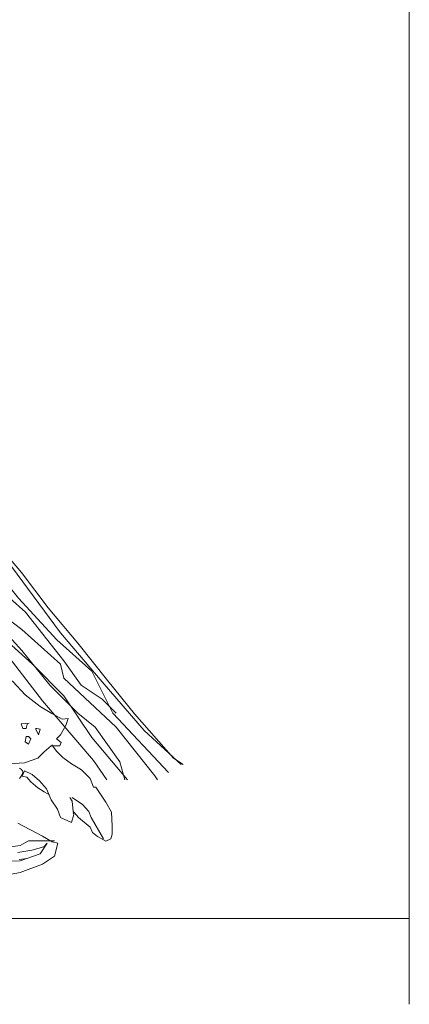
# Model space of a CAD drawing. Units: inches. Extents: x -17 to 1735, y -531 to 60.
# Tile 24 of 27: x 1734.80712 to 1734.81148, y -150.21559 to -150.20455. Entities that reach past the tile are written whole.
import ezdxf

# ---------------------------------------------------------------- set-up
doc = ezdxf.new("R2010")
doc.units = ezdxf.units.IN
doc.header["$MEASUREMENT"] = 0
doc.layers.add('A-FURN', color=242, linetype='Continuous', lineweight=18, true_color=0xcd2027)

# ---------------------------------------------------------------- blocks, each defined once
blk = doc.blocks.new('childrens_room_2')
for p, q in [((73.63163, 54.17766), (73.63163, 54.90289)), ((73.63163, 54.20212), (73.14631, 54.20212))]:
    blk.add_line(p, q)
for points in [[(73.45448, 54.41111), (73.45858, 54.40576), (73.46299, 54.39757), (73.46709, 54.3897), (73.47119, 54.38214), (73.47718, 54.3708), (73.48475, 54.36198), (73.49042, 54.35222), (73.49894, 54.33301), (73.50907, 54.3176), (73.5138, 54.30941), (73.52137, 54.3006), (73.52894, 54.29052), (73.53745, 54.28044), (73.54596, 54.26974), (73.55353, 54.26029), (73.56456, 54.24769), (73.56734, 54.24595)], [(73.42106, 54.40855), (73.42295, 54.40603), (73.42737, 54.39974), (73.43241, 54.39344), (73.44093, 54.38273), (73.44629, 54.37958), (73.45259, 54.37423), (73.45701, 54.36919), (73.46079, 54.36226), (73.46489, 54.35502), (73.46741, 54.34746), (73.46962, 54.34116), (73.47183, 54.33487), (73.47592, 54.32731), (73.48002, 54.32196), (73.48009, 54.32041), (73.48639, 54.31506), (73.49396, 54.30246), (73.50216, 54.29239), (73.51603, 54.27885), (73.52738, 54.26405), (73.54189, 54.24704), (73.54565, 54.24155)], [(73.42509, 54.40843), (73.43702, 54.39652), (73.44994, 54.38163), (73.46088, 54.36376), (73.46783, 54.34887), (73.47479, 54.34291), (73.48175, 54.32505), (73.4887, 54.31512), (73.49765, 54.30321), (73.50461, 54.29527), (73.51355, 54.28435), (73.52448, 54.27442), (73.53343, 54.26549), (73.54138, 54.25358), (73.55157, 54.24155)], [(73.441, 54.40843), (73.44795, 54.40148), (73.45392, 54.38758), (73.46286, 54.37369), (73.46883, 54.35979), (73.47678, 54.34688), (73.48572, 54.33497), (73.49367, 54.32008), (73.5056, 54.30619), (73.51355, 54.2903), (73.5215, 54.28435), (73.53244, 54.27442), (73.53343, 54.27045), (73.54834, 54.25655), (73.55927, 54.24266), (73.5601, 54.24155)], [(73.44696, 54.40942), (73.45988, 54.3985), (73.46883, 54.37369), (73.47578, 54.36277), (73.48473, 54.34887), (73.49268, 54.33497), (73.50163, 54.32108), (73.50858, 54.30817), (73.52051, 54.29328), (73.53144, 54.28137), (73.54138, 54.27244), (73.54734, 54.26052), (73.56316, 54.2436)], [(73.45094, 54.40843), (73.45789, 54.40049), (73.46584, 54.38858), (73.4738, 54.36277), (73.46982, 54.37766), (73.47877, 54.36475), (73.48572, 54.35086), (73.49268, 54.34192), (73.50063, 54.32703), (73.50958, 54.31611), (73.51852, 54.30222), (73.53244, 54.28336), (73.54436, 54.26946), (73.55629, 54.25556), (73.56679, 54.24595)], [(73.43802, 54.40644), (73.44895, 54.39354), (73.46783, 54.35582), (73.4738, 54.34788), (73.48175, 54.332), (73.4897, 54.32008), (73.49566, 54.31016), (73.50262, 54.30023), (73.51057, 54.2903), (73.5215, 54.27839), (73.52945, 54.26847), (73.53741, 54.26052), (73.54238, 54.25655), (73.54933, 54.24663), (73.55079, 54.24155)], [(73.47578, 54.35185), (73.48672, 54.33696), (73.49765, 54.32306), (73.50262, 54.31115), (73.51355, 54.29725), (73.5225, 54.28931), (73.53343, 54.27541), (73.5384, 54.26847), (73.54436, 54.26449), (73.54834, 54.26052)], [(73.52083, 54.24491), (73.52111, 54.2447), (73.52135, 54.2445), (73.52153, 54.24428), (73.52166, 54.24407), (73.52173, 54.24385), (73.52174, 54.24362), (73.52169, 54.24339), (73.5216, 54.24314), (73.52146, 54.24288), (73.52128, 54.24259), (73.52107, 54.24229), (73.52082, 54.24197)], [(73.51778, 54.27017), (73.51889, 54.26951), (73.52246, 54.26572), (73.52669, 54.26238), (73.53003, 54.26038), (73.53293, 54.25882), (73.53471, 54.25904), (73.53404, 54.25704), (73.53248, 54.25437), (73.53137, 54.25326), (73.53271, 54.25214), (73.53226, 54.25125), (73.52981, 54.25125), (73.5278, 54.24947), (73.52602, 54.24769), (73.52223, 54.24636), (73.51778, 54.24613)], [(73.52036, 54.22921), (73.52739, 54.22553), (73.53007, 54.22386), (73.53174, 54.22352), (73.53074, 54.21984), (73.52739, 54.2175), (73.52103, 54.21516), (73.514, 54.21383)], [(73.52036, 54.22085), (73.52438, 54.22152), (73.52773, 54.22252), (73.52873, 54.22352), (73.52672, 54.22051), (73.52103, 54.21851), (73.513, 54.21817)], [(73.5207, 54.21884), (73.52304, 54.21918)], [(73.52357, 54.25771), (73.52134, 54.25749), (73.52179, 54.25615), (73.52268, 54.25615), (73.52312, 54.25771)], [(73.52357, 54.25392), (73.52268, 54.25392), (73.52246, 54.25237), (73.52335, 54.2517), (73.52402, 54.25326), (73.52335, 54.25392)], [(73.52535, 54.25615), (73.52624, 54.25437), (73.52669, 54.25593), (73.5258, 54.25615), (73.52558, 54.25615)], [(73.53003, 54.25148), (73.53137, 54.2497), (73.53315, 54.24792), (73.5356, 54.24613), (73.5385, 54.24435), (73.54095, 54.24191), (73.54184, 54.23946), (73.54251, 54.23946), (73.54541, 54.23523), (73.54697, 54.23233), (73.54719, 54.22833), (73.54719, 54.2261), (73.54675, 54.22477), (73.54541, 54.2241), (73.54296, 54.22543), (73.54162, 54.22655), (73.54095, 54.22811), (73.53761, 54.23078), (73.5365, 54.23211), (73.53605, 54.23211), (73.53627, 54.23167), (73.5356, 54.22944), (73.53248, 54.23078), (73.53159, 54.23322), (73.52981, 54.2359), (73.52847, 54.23901), (73.52647, 54.24124), (73.52446, 54.24302), (73.52223, 54.24413), (73.52156, 54.24257), (73.5229, 54.24235), (73.52402, 54.24102), (73.52602, 54.23923), (73.5278, 54.23812), (73.52936, 54.23723)], [(73.53516, 54.23656), (73.53583, 54.23545), (73.53605, 54.23256), (73.53672, 54.23189)], [(73.53583, 54.23656), (73.53872, 54.23456), (73.54051, 54.23256), (73.54118, 54.23078), (73.54474, 54.22477)], [(73.47784, 54.21817), (73.4919, 54.22018), (73.50195, 54.22018), (73.50898, 54.22185), (73.51634, 54.22219), (73.52103, 54.22285), (73.52337, 54.22419), (73.52773, 54.22419), (73.53074, 54.22419)]]:
    blk.add_lwpolyline(points)

msp = doc.modelspace()

# ---------------------------------------------------------------- block references
at = {"layer": 'A-FURN', "xscale": 0.0393700787401575, "yscale": 0.0393700787401575, "zscale": 0.0393700787401575}
msp.add_blockref('childrens_room_2', (1731.912601, -152.348565), dxfattribs=at)

doc.saveas('drawing.dxf')
